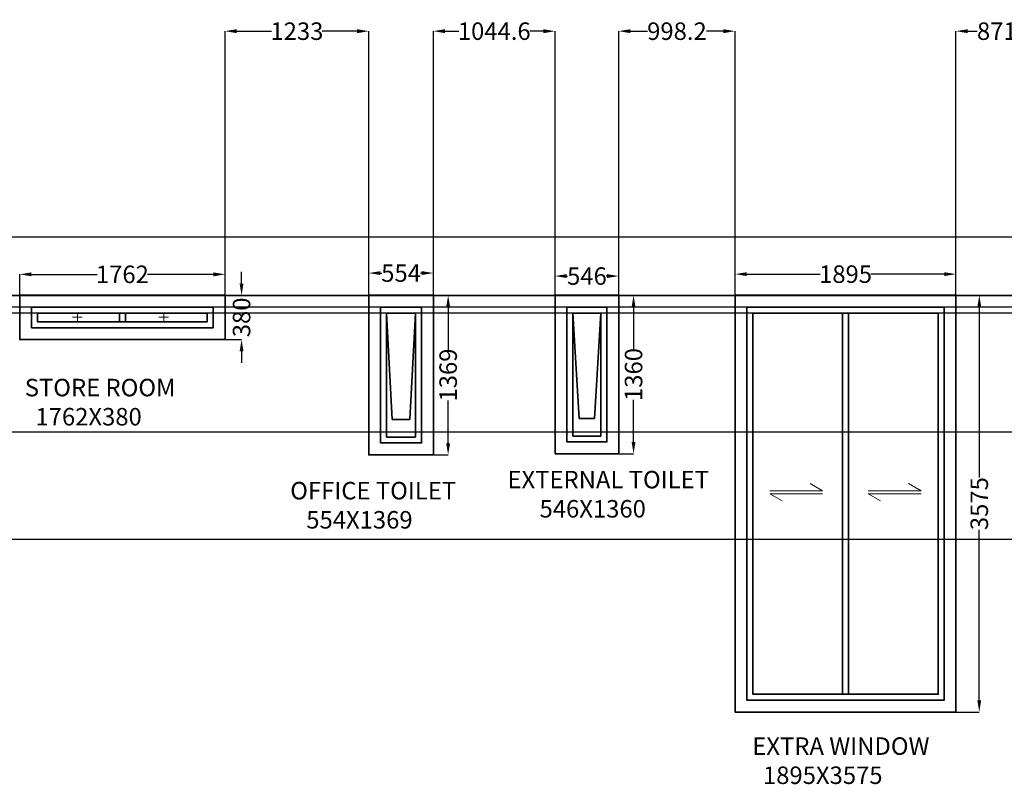
# Model space of a CAD drawing. Units: millimetres. Extents: x 16338 to 57165, y -4429 to 26237.
# Tile 3 of 6: x 32038 to 40486, y 2640 to 9199. Entities that reach past the tile are written whole.
import ezdxf

# ---------------------------------------------------------------- set-up
doc = ezdxf.new("R2010")
doc.units = ezdxf.units.MM
doc.header["$MEASUREMENT"] = 0
for name, color, linetype, lineweight in [('A-ANNO-DIMS', 5, 'Continuous', 18), ('A-ANNO-SYMB', 4, 'Continuous', 18), ('A-ANNO-TEXT', 3, 'Continuous', 18), ('A-ELEV', 8, 'Continuous', 25), ('A-GLAZ', 7, 'Continuous', 35)]:
    doc.layers.add(name, color=color, linetype=linetype, lineweight=lineweight)
doc.styles.get("Standard").update_dxf_attribs({"font": 'arial.ttf'})
doc.dimstyles.get("Standard").update_dxf_attribs({"dimtxt": 150, "dimasz": 100, "dimexe": 0.18, "dimexo": 0.0625, "dimgap": 0.09, "dimtad": 0, "dimdec": 0, "dimzin": 0, "dimdsep": 46, "dimtxsty": 'Standard', "dimcen": 0.09, "dimadec": 0, "dimazin": 0, "dimtfac": 1, "dimtdec": 0, "dimtofl": 0, "dimtmove": 0, "dimatfit": 3, "dimfxl": 1, "dimtolj": 1, "dimtzin": 0, "dimarcsym": 0})

# ---------------------------------------------------------------- blocks, each defined once
blk = doc.blocks.new('*D59')
at = {"layer": 'A-ANNO-DIMS', "color": 0, "lineweight": -2, "transparency": 16777216}
for p, q in [((32038.1, 6835.2), (32038.1, 7014.4)), ((32138.1, 7014.2), (32702.9, 7014.2)), ((33700.1, 7014.2), (33135.4, 7014.2)), ((33800.1, 6835.2), (33800.1, 7014.4))]:
    blk.add_line(p, q, dxfattribs=at)
at = {"layer": 'A-ANNO-DIMS', "color": 0, "transparency": 16777216}
for points in [[(32138.1, 7030.9), (32138.1, 6997.5), (32038.1, 7014.2)], [(33700.1, 7030.9), (33700.1, 6997.5), (33800.1, 7014.2)]]:
    blk.add_solid(points, dxfattribs=at)
at = {"layer": 'Defpoints', "color": 0, "transparency": 16777216}
for p in [(33800.1, 7014.2), (32038.1, 6835.1), (33800.1, 6835.1)]:
    blk.add_point(p, dxfattribs=at)
at = {"layer": 'A-ANNO-DIMS', "color": 0, "transparency": 16777216, "insert": (32919.1, 7014.2), "char_height": 150, "attachment_point": 5}
blk.add_mtext('\\A1;1762', dxfattribs=at)
blk = doc.blocks.new('*D60')
at = {"layer": 'A-ANNO-DIMS', "color": 0, "lineweight": -2, "transparency": 16777216}
for p, q in [((33941.5, 6935.1), (33941.5, 7035.1)), ((33800.2, 6835.1), (33941.7, 6835.1)), ((33800.2, 6455.1), (33941.7, 6455.1)), ((33941.5, 6355.1), (33941.5, 6255.1))]:
    blk.add_line(p, q, dxfattribs=at)
at = {"layer": 'A-ANNO-DIMS', "color": 0, "transparency": 16777216}
for points in [[(33924.9, 6935.1), (33958.2, 6935.1), (33941.5, 6835.1)], [(33924.9, 6355.1), (33958.2, 6355.1), (33941.5, 6455.1)]]:
    blk.add_solid(points, dxfattribs=at)
at = {"layer": 'Defpoints', "color": 0, "transparency": 16777216}
for p in [(33800.1, 6835.1), (33800.1, 6455.1), (33941.5, 6455.1)]:
    blk.add_point(p, dxfattribs=at)
at = {"layer": 'A-ANNO-DIMS', "color": 0, "transparency": 16777216, "insert": (33941.5, 6645.1), "char_height": 150, "attachment_point": 5, "rotation": 90}
blk.add_mtext('\\A1;380', dxfattribs=at)
blk = doc.blocks.new('*D61')
at = {"layer": 'A-ANNO-DIMS', "color": 0, "lineweight": -2, "transparency": 16777216}
for p, q in [((35033.2, 6835.2), (35033.2, 7025.4)), ((35133.2, 7025.2), (35144.7, 7025.2)), ((35487.2, 7025.2), (35475.7, 7025.2)), ((35587.2, 6835.2), (35587.2, 7025.4))]:
    blk.add_line(p, q, dxfattribs=at)
at = {"layer": 'A-ANNO-DIMS', "color": 0, "transparency": 16777216}
for points in [[(35133.2, 7041.9), (35133.2, 7008.5), (35033.2, 7025.2)], [(35487.2, 7041.9), (35487.2, 7008.5), (35587.2, 7025.2)]]:
    blk.add_solid(points, dxfattribs=at)
at = {"layer": 'Defpoints', "color": 0, "transparency": 16777216}
for p in [(35587.2, 7025.2), (35033.2, 6835.1), (35587.2, 6835.1)]:
    blk.add_point(p, dxfattribs=at)
at = {"layer": 'A-ANNO-DIMS', "color": 0, "transparency": 16777216, "insert": (35310.2, 7025.2), "char_height": 150, "attachment_point": 5}
blk.add_mtext('\\A1;554', dxfattribs=at)
blk = doc.blocks.new('*D62')
at = {"layer": 'A-ANNO-DIMS', "color": 0, "lineweight": -2, "transparency": 16777216}
for p, q in [((35587.2, 6835.1), (35714.3, 6835.1)), ((35714.1, 6735.1), (35714.1, 6367.8)), ((35714.1, 5566.1), (35714.1, 5933.4)), ((35587.2, 5466.1), (35714.3, 5466.1))]:
    blk.add_line(p, q, dxfattribs=at)
at = {"layer": 'A-ANNO-DIMS', "color": 0, "transparency": 16777216}
for points in [[(35697.5, 6735.1), (35730.8, 6735.1), (35714.1, 6835.1)], [(35697.5, 5566.1), (35730.8, 5566.1), (35714.1, 5466.1)]]:
    blk.add_solid(points, dxfattribs=at)
at = {"layer": 'Defpoints', "color": 0, "transparency": 16777216}
for p in [(35587.2, 6835.1), (35587.2, 5466.1), (35714.1, 5466.1)]:
    blk.add_point(p, dxfattribs=at)
at = {"layer": 'A-ANNO-DIMS', "color": 0, "transparency": 16777216, "insert": (35714.1, 6150.6), "char_height": 150, "attachment_point": 5, "rotation": 90}
blk.add_mtext('\\A1;1369', dxfattribs=at)
blk = doc.blocks.new('*D63')
at = {"layer": 'A-ANNO-DIMS', "color": 0, "lineweight": -2, "transparency": 16777216}
for p, q in [((36631.8, 6835.2), (36631.8, 6999.8)), ((36731.8, 6999.6), (36739, 6999.6)), ((37077.8, 6999.6), (37070.5, 6999.6)), ((37177.8, 6835.2), (37177.8, 6999.8))]:
    blk.add_line(p, q, dxfattribs=at)
at = {"layer": 'A-ANNO-DIMS', "color": 0, "transparency": 16777216}
for points in [[(36731.8, 7016.3), (36731.8, 6983), (36631.8, 6999.6)], [(37077.8, 7016.3), (37077.8, 6983), (37177.8, 6999.6)]]:
    blk.add_solid(points, dxfattribs=at)
at = {"layer": 'Defpoints', "color": 0, "transparency": 16777216}
for p in [(37177.8, 6999.6), (36631.8, 6835.1), (37177.8, 6835.1)]:
    blk.add_point(p, dxfattribs=at)
at = {"layer": 'A-ANNO-DIMS', "color": 0, "transparency": 16777216, "insert": (36904.8, 6999.6), "char_height": 150, "attachment_point": 5}
blk.add_mtext('\\A1;546', dxfattribs=at)
blk = doc.blocks.new('*D64')
at = {"layer": 'A-ANNO-DIMS', "color": 0, "lineweight": -2, "transparency": 16777216}
for p, q in [((37177.8, 6835.1), (37304.9, 6835.1)), ((37304.7, 6735.1), (37304.7, 6371.9)), ((37304.7, 5575.1), (37304.7, 5938.4)), ((37177.8, 5475.1), (37304.9, 5475.1))]:
    blk.add_line(p, q, dxfattribs=at)
at = {"layer": 'A-ANNO-DIMS', "color": 0, "transparency": 16777216}
for points in [[(37288, 6735.1), (37321.4, 6735.1), (37304.7, 6835.1)], [(37288, 5575.1), (37321.4, 5575.1), (37304.7, 5475.1)]]:
    blk.add_solid(points, dxfattribs=at)
at = {"layer": 'Defpoints', "color": 0, "transparency": 16777216}
for p in [(37177.8, 6835.1), (37177.8, 5475.1), (37304.7, 5475.1)]:
    blk.add_point(p, dxfattribs=at)
at = {"layer": 'A-ANNO-DIMS', "color": 0, "transparency": 16777216, "insert": (37304.7, 6155.1), "char_height": 150, "attachment_point": 5, "rotation": 90}
blk.add_mtext('\\A1;1360', dxfattribs=at)
blk = doc.blocks.new('*D65')
at = {"layer": 'A-ANNO-DIMS', "color": 0, "lineweight": -2, "transparency": 16777216}
for p, q in [((38176, 6835.2), (38176, 7016.2)), ((38276, 7016.1), (38905.9, 7016.1)), ((39971, 7016.1), (39341, 7016.1)), ((40071, 6835.2), (40071, 7016.2))]:
    blk.add_line(p, q, dxfattribs=at)
at = {"layer": 'A-ANNO-DIMS', "color": 0, "transparency": 16777216}
for points in [[(38276, 7032.7), (38276, 6999.4), (38176, 7016.1)], [(39971, 7032.7), (39971, 6999.4), (40071, 7016.1)]]:
    blk.add_solid(points, dxfattribs=at)
at = {"layer": 'Defpoints', "color": 0, "transparency": 16777216}
for p in [(40071, 7016.1), (38176, 6835.1), (40071, 6835.1)]:
    blk.add_point(p, dxfattribs=at)
at = {"layer": 'A-ANNO-DIMS', "color": 0, "transparency": 16777216, "insert": (39123.5, 7016.1), "char_height": 150, "attachment_point": 5}
blk.add_mtext('\\A1;1895', dxfattribs=at)
blk = doc.blocks.new('*D66')
at = {"layer": 'A-ANNO-DIMS', "color": 0, "lineweight": -2, "transparency": 16777216}
for p, q in [((40071, 6835.1), (40271.1, 6835.1)), ((40270.9, 6735.1), (40270.9, 5272.2)), ((40270.9, 3360.1), (40270.9, 4823)), ((40071, 3260.1), (40271.1, 3260.1))]:
    blk.add_line(p, q, dxfattribs=at)
at = {"layer": 'A-ANNO-DIMS', "color": 0, "transparency": 16777216}
for points in [[(40254.2, 6735.1), (40287.6, 6735.1), (40270.9, 6835.1)], [(40254.2, 3360.1), (40287.6, 3360.1), (40270.9, 3260.1)]]:
    blk.add_solid(points, dxfattribs=at)
at = {"layer": 'Defpoints', "color": 0, "transparency": 16777216}
for p in [(40071, 6835.1), (40071, 3260.1), (40270.9, 3260.1)]:
    blk.add_point(p, dxfattribs=at)
at = {"layer": 'A-ANNO-DIMS', "color": 0, "transparency": 16777216, "insert": (40270.9, 5047.6), "char_height": 150, "attachment_point": 5, "rotation": 90}
blk.add_mtext('\\A1;3575', dxfattribs=at)
blk = doc.blocks.new('SLIDE-ARROW-L')
for p, q in [((454.2, 0), (346.9, 62)), ((0, 0), (454.2, 0))]:
    blk.add_line(p, q)
blk = doc.blocks.new('*D113')
at = {"layer": 'A-ANNO-DIMS', "color": 0, "lineweight": -2, "transparency": 16777216}
for p, q in [((33800.1, 6835.2), (33800.1, 9100.3)), ((33900.1, 9100.1), (34199.6, 9100.1)), ((34933.2, 9100.1), (34633.7, 9100.1)), ((35033.2, 6835.2), (35033.2, 9100.3))]:
    blk.add_line(p, q, dxfattribs=at)
at = {"layer": 'A-ANNO-DIMS', "color": 0, "transparency": 16777216}
for points in [[(33900.1, 9116.8), (33900.1, 9083.4), (33800.1, 9100.1)], [(34933.2, 9116.8), (34933.2, 9083.4), (35033.2, 9100.1)]]:
    blk.add_solid(points, dxfattribs=at)
at = {"layer": 'Defpoints', "color": 0, "transparency": 16777216}
for p in [(35033.2, 9100.1), (33800.1, 6835.1), (35033.2, 6835.1)]:
    blk.add_point(p, dxfattribs=at)
at = {"layer": 'A-ANNO-DIMS', "color": 0, "transparency": 16777216, "insert": (34416.7, 9100.1), "char_height": 150, "attachment_point": 5}
blk.add_mtext('\\A1;1233', dxfattribs=at)
blk = doc.blocks.new('*D114')
at = {"layer": 'A-ANNO-DIMS', "color": 0, "lineweight": -2, "transparency": 16777216}
for p, q in [((35587.2, 6835.2), (35587.2, 9100.3)), ((35687.2, 9100.1), (35805.1, 9100.1)), ((36531.8, 9100.1), (36413.8, 9100.1)), ((36631.8, 6835.2), (36631.8, 9100.3))]:
    blk.add_line(p, q, dxfattribs=at)
at = {"layer": 'A-ANNO-DIMS', "color": 0, "transparency": 16777216}
for points in [[(35687.2, 9116.8), (35687.2, 9083.4), (35587.2, 9100.1)], [(36531.8, 9116.8), (36531.8, 9083.4), (36631.8, 9100.1)]]:
    blk.add_solid(points, dxfattribs=at)
at = {"layer": 'Defpoints', "color": 0, "transparency": 16777216}
for p in [(36631.8, 9100.1), (35587.2, 6835.1), (36631.8, 6835.1)]:
    blk.add_point(p, dxfattribs=at)
at = {"layer": 'A-ANNO-DIMS', "color": 0, "transparency": 16777216, "insert": (36109.5, 9100.1), "char_height": 150, "attachment_point": 5}
blk.add_mtext('\\A1;1044.6', dxfattribs=at)
blk = doc.blocks.new('*D115')
at = {"layer": 'A-ANNO-DIMS', "color": 0, "lineweight": -2, "transparency": 16777216}
for p, q in [((37177.8, 6835.2), (37177.8, 9100.3)), ((37277.8, 9100.1), (37424.5, 9100.1)), ((38076, 9100.1), (37929.3, 9100.1)), ((38176, 6835.2), (38176, 9100.3))]:
    blk.add_line(p, q, dxfattribs=at)
at = {"layer": 'A-ANNO-DIMS', "color": 0, "transparency": 16777216}
for points in [[(37277.8, 9116.8), (37277.8, 9083.4), (37177.8, 9100.1)], [(38076, 9116.8), (38076, 9083.4), (38176, 9100.1)]]:
    blk.add_solid(points, dxfattribs=at)
at = {"layer": 'Defpoints', "color": 0, "transparency": 16777216}
for p in [(38176, 9100.1), (37177.8, 6835.1), (38176, 6835.1)]:
    blk.add_point(p, dxfattribs=at)
at = {"layer": 'A-ANNO-DIMS', "color": 0, "transparency": 16777216, "insert": (37676.9, 9100.1), "char_height": 150, "attachment_point": 5}
blk.add_mtext('\\A1;998.2', dxfattribs=at)
blk = doc.blocks.new('*D116')
at = {"layer": 'A-ANNO-DIMS', "color": 0, "lineweight": -2, "transparency": 16777216}
for p, q in [((40071, 6835.2), (40071, 9100.3)), ((40171, 9100.1), (40254, 9100.1)), ((40842.1, 9100.1), (40759.1, 9100.1)), ((40942.1, 6834.3), (40942.1, 9100.3))]:
    blk.add_line(p, q, dxfattribs=at)
at = {"layer": 'A-ANNO-DIMS', "color": 0, "transparency": 16777216}
for points in [[(40171, 9116.8), (40171, 9083.4), (40071, 9100.1)], [(40842.1, 9116.8), (40842.1, 9083.4), (40942.1, 9100.1)]]:
    blk.add_solid(points, dxfattribs=at)
at = {"layer": 'Defpoints', "color": 0, "transparency": 16777216}
for p in [(40942.1, 9100.1), (40071, 6835.1), (40942.1, 6834.2)]:
    blk.add_point(p, dxfattribs=at)
at = {"layer": 'A-ANNO-DIMS', "color": 0, "transparency": 16777216, "insert": (40506.6, 9100.1), "char_height": 150, "attachment_point": 5}
blk.add_mtext('\\A1;871.2', dxfattribs=at)
blk = doc.blocks.new('*D126')
at = {"layer": 'A-ANNO-DIMS', "color": 0, "lineweight": -2, "transparency": 16777216}
for p, q in [((52647.9, 6935.1), (52647.9, 7035.1)), ((23824.7, 6835.1), (52648.1, 6835.1)), ((23724.7, 6735.1), (52648.1, 6735.1)), ((52647.9, 6635.1), (52647.9, 6535.1))]:
    blk.add_line(p, q, dxfattribs=at)
at = {"layer": 'A-ANNO-DIMS', "color": 0, "transparency": 16777216}
for points in [[(52631.2, 6935.1), (52664.6, 6935.1), (52647.9, 6835.1)], [(52631.2, 6635.1), (52664.6, 6635.1), (52647.9, 6735.1)]]:
    blk.add_solid(points, dxfattribs=at)
at = {"layer": 'Defpoints', "color": 0, "transparency": 16777216}
for p in [(23824.6, 6835.1), (23724.6, 6735.1), (52647.9, 6735.1)]:
    blk.add_point(p, dxfattribs=at)
at = {"layer": 'A-ANNO-DIMS', "color": 0, "transparency": 16777216, "insert": (52647.9, 6376.6), "char_height": 150, "attachment_point": 5, "rotation": 90}
blk.add_mtext('\\A1;100', dxfattribs=at)
blk = doc.blocks.new('*D127')
at = {"layer": 'A-ANNO-DIMS', "color": 0, "lineweight": -2, "transparency": 16777216}
for p, q in [((52647.9, 6835.1), (52647.9, 6935.1)), ((23673.9, 6684.3), (52648.1, 6684.3)), ((23724.7, 6735.1), (52648.1, 6735.1)), ((52647.9, 6584.3), (52647.9, 6484.3))]:
    blk.add_line(p, q, dxfattribs=at)
at = {"layer": 'A-ANNO-DIMS', "color": 0, "transparency": 16777216}
for points in [[(52631.2, 6835.1), (52664.6, 6835.1), (52647.9, 6735.1)], [(52631.2, 6584.3), (52664.6, 6584.3), (52647.9, 6684.3)]]:
    blk.add_solid(points, dxfattribs=at)
at = {"layer": 'Defpoints', "color": 0, "transparency": 16777216}
for p in [(23673.8, 6684.3), (23724.6, 6735.1), (52647.9, 6684.3)]:
    blk.add_point(p, dxfattribs=at)
at = {"layer": 'A-ANNO-DIMS', "color": 0, "transparency": 16777216, "insert": (52647.9, 6289.2), "char_height": 150, "attachment_point": 5, "rotation": 90}
blk.add_mtext('\\A1;50.8', dxfattribs=at)
blk = doc.blocks.new('*D132')
at = {"layer": 'A-ANNO-DIMS', "color": 0, "lineweight": -2, "transparency": 16777216}
for p, q in [((23673.9, 5663.2), (52648.1, 5663.2)), ((52647.9, 5563.2), (52647.9, 5441.3)), ((52647.9, 4842), (52647.9, 4963.9)), ((23615.6, 4742), (52648.1, 4742))]:
    blk.add_line(p, q, dxfattribs=at)
at = {"layer": 'A-ANNO-DIMS', "color": 0, "transparency": 16777216}
for points in [[(52631.2, 5563.2), (52664.6, 5563.2), (52647.9, 5663.2)], [(52631.2, 4842), (52664.6, 4842), (52647.9, 4742)]]:
    blk.add_solid(points, dxfattribs=at)
at = {"layer": 'Defpoints', "color": 0, "transparency": 16777216}
for p in [(23673.8, 5663.2), (52647.9, 5663.2), (23615.6, 4742)]:
    blk.add_point(p, dxfattribs=at)
at = {"layer": 'A-ANNO-DIMS', "color": 0, "transparency": 16777216, "insert": (52647.9, 5202.6), "char_height": 150, "attachment_point": 5, "rotation": 90}
blk.add_mtext('\\A1;921.1', dxfattribs=at)

msp = doc.modelspace()

# ---------------------------------------------------------------- linework, layer by layer
at = {"layer": 'A-ANNO-SYMB'}
for p, q in [((32492.52, 6645.62), (32575.1, 6645.62)), ((32533.81, 6615.33), (32533.81, 6672.29)), ((33232.11, 6645.62), (33314.69, 6645.62)), ((33273.4, 6615.33), (33273.4, 6672.29))]:
    msp.add_line(p, q, dxfattribs=at)
at = {"layer": 'A-ELEV'}
for p, q in [((18209.23, 7335.1), (50757.08, 7335.1)), ((18201.83, 6834.85), (50882.91, 6829.39))]:
    msp.add_line(p, q, dxfattribs=at)
at = {"layer": 'A-GLAZ'}
for p, q in [((32893.73, 6682.7), (32893.73, 6607.5)), ((32944.53, 6682.7), (32944.53, 6607.5)), ((35185.57, 6682.7), (35434.77, 6682.7)), ((35185.57, 5618.5), (35185.57, 6682.7)), ((35185.57, 6682.7), (35234.02, 5768.5)), ((35434.77, 6682.7), (35386.33, 5768.5)), ((35434.77, 6682.7), (35434.77, 5618.5)), ((36784.18, 6682.7), (37025.38, 6682.7)), ((36784.18, 5627.5), (36784.18, 6682.7)), ((36784.18, 6682.7), (36839.44, 5777.5)), ((37025.38, 6682.7), (36970.12, 5777.5)), ((37025.38, 6682.7), (37025.38, 5627.5)), ((39098.07, 6682.7), (39098.07, 3412.5)), ((39148.87, 6682.7), (39148.87, 3412.5)), ((35386.33, 5768.5), (35234.02, 5768.5)), ((36970.12, 5777.5), (36839.44, 5777.5)), ((35434.77, 5618.5), (35185.57, 5618.5)), ((37025.38, 5627.5), (36784.18, 5627.5))]:
    msp.add_line(p, q, dxfattribs=at)
for points in [[(32038.13, 6835.1), (33800.13, 6835.1), (33800.13, 6455.1), (32038.13, 6455.1)], [(35033.17, 6835.1), (35587.17, 6835.1), (35587.17, 5466.1), (35033.17, 5466.1)], [(36631.78, 6835.1), (37177.78, 6835.1), (37177.78, 5475.1), (36631.78, 5475.1)], [(38175.97, 6835.1), (40070.97, 6835.1), (40070.97, 3260.1), (38175.97, 3260.1)], [(32139.73, 6733.5), (33698.53, 6733.5), (33698.53, 6556.7), (32139.73, 6556.7)], [(32190.53, 6682.7), (33647.73, 6682.7), (33647.73, 6607.5), (32190.53, 6607.5)], [(35134.77, 6733.5), (35485.57, 6733.5), (35485.57, 5567.7), (35134.77, 5567.7)], [(36733.38, 6733.5), (37076.18, 6733.5), (37076.18, 5576.7), (36733.38, 5576.7)], [(38277.57, 6733.5), (39969.37, 6733.5), (39969.37, 3361.7), (38277.57, 3361.7)], [(38328.37, 6682.7), (39918.57, 6682.7), (39918.57, 3412.5), (38328.37, 3412.5)]]:
    msp.add_lwpolyline(points, close=True, dxfattribs=at)

# ---------------------------------------------------------------- block references
at = {"layer": 'A-ANNO-SYMB'}
for p in [(38472.73, 5156.9), (39316.72, 5156.9)]:
    msp.add_blockref('SLIDE-ARROW-L', p, dxfattribs=at)
at = {"layer": 'A-ANNO-SYMB', "rotation": 180}
for p in [(38926.93, 5132.25), (39770.92, 5132.25)]:
    msp.add_blockref('SLIDE-ARROW-L', p, dxfattribs=at)

# ---------------------------------------------------------------- texts
at = {"layer": 'A-ANNO-TEXT', "char_height": 150, "attachment_point": 1}
for s, insert in [('STORE ROOM\\P  1762X380', (32081.77, 6118.08)), ('EXTERNAL TOILET\\P      546X1360', (36223.1, 5328.43)), ('OFFICE TOILET\\P   554X1369', (34359.36, 5233.87)), ('EXTRA WINDOW\\P  1895X3575', (38323.32, 3042.82))]:
    msp.add_mtext_dynamic_manual_height_columns(s, width=7094.9176, gutter_width=1, heights=[0], dxfattribs=dict(at, insert=insert))

# ---------------------------------------------------------------- dimensions: what is measured, and where the dimension line sits
at = {"layer": 'A-ANNO-DIMS'}
for base, p1, p2, override, picture, middle in [((35033.17, 9100.1), (33800.13, 6835.1), (35033.17, 6835.1), {"dimdec": 0, "dimlfac": 1, "dimrnd": 0, "dimzin": 0, "dimdsep": 46, "dimlunit": 2}, '*D113', (34416.65, 9100.1)), ((36631.78, 9100.1), (35587.17, 6835.1), (36631.78, 6835.1), {"dimdec": 1, "dimlfac": 1, "dimrnd": 0, "dimzin": 0, "dimdsep": 46, "dimlunit": 2}, '*D114', (36109.48, 9100.1)), ((38175.97, 9100.1), (37177.78, 6835.1), (38175.97, 6835.1), {"dimdec": 1, "dimlfac": 1, "dimrnd": 0, "dimzin": 0, "dimdsep": 46, "dimlunit": 2}, '*D115', (37676.87, 9100.1)), ((40942.14, 9100.1), (40070.97, 6835.1), (40942.14, 6834.2), {"dimdec": 1, "dimlfac": 1, "dimrnd": 0, "dimzin": 0, "dimdsep": 46, "dimlunit": 2}, '*D116', (40506.55, 9100.1)), ((33800.13, 7014.2), (32038.13, 6835.1), (33800.13, 6835.1), {"dimclrd": 0, "dimclre": 0, "dimclrt": 0}, '*D59', (32919.13, 7014.2)), ((35587.17, 7025.19), (35033.17, 6835.1), (35587.17, 6835.1), {"dimclrd": 0, "dimclre": 0, "dimclrt": 0}, '*D61', (35310.17, 7025.19)), ((37177.78, 6999.64), (36631.78, 6835.1), (37177.78, 6835.1), {"dimclrd": 0, "dimclre": 0, "dimclrt": 0}, '*D63', (36904.78, 6999.64)), ((40070.97, 7016.05), (38175.97, 6835.1), (40070.97, 6835.1), {"dimclrd": 0, "dimclre": 0, "dimclrt": 0}, '*D65', (39123.47, 7016.05))]:
    dim = msp.add_linear_dim(base=base, p1=p1, p2=p2, dimstyle='Standard', override=override, dxfattribs=at)
    dim.commit()
    dim.dimension.update_dxf_attribs({"geometry": picture, "text_midpoint": middle})
for base, p1, p2, override, picture, middle in [((52647.91, 6735.1), (23824.59, 6835.1), (23724.59, 6735.1), {"dimdec": 0, "dimlfac": 1, "dimrnd": 0, "dimzin": 0, "dimdsep": 46, "dimlunit": 2}, '*D126', (52647.91, 6376.62)), ((33941.55, 6455.1), (33800.13, 6835.1), (33800.13, 6455.1), {"dimclrd": 0, "dimclre": 0, "dimclrt": 0}, '*D60', (33941.55, 6645.1)), ((52647.91, 6684.3), (23724.59, 6735.1), (23673.79, 6684.3), {"dimdec": 1, "dimlfac": 1, "dimrnd": 0, "dimzin": 0, "dimdsep": 46, "dimlunit": 2}, '*D127', (52647.91, 6289.25)), ((35714.12, 5466.1), (35587.17, 6835.1), (35587.17, 5466.1), {"dimclrd": 0, "dimclre": 0, "dimclrt": 0}, '*D62', (35714.12, 6150.6)), ((37304.7, 5475.1), (37177.78, 6835.1), (37177.78, 5475.1), {"dimclrd": 0, "dimclre": 0, "dimclrt": 0}, '*D64', (37304.7, 6155.1)), ((40270.89, 3260.1), (40070.97, 6835.1), (40070.97, 3260.1), {"dimclrd": 0, "dimclre": 0, "dimclrt": 0}, '*D66', (40270.89, 5047.6)), ((52647.91, 5663.17), (23615.55, 4742.04), (23673.79, 5663.17), {"dimdec": 1, "dimlfac": 1, "dimrnd": 0, "dimzin": 0, "dimdsep": 46, "dimlunit": 2}, '*D132', (52647.91, 5202.6))]:
    dim = msp.add_linear_dim(base=base, p1=p1, p2=p2, angle=90, dimstyle='Standard', override=override, dxfattribs=at)
    dim.commit()
    dim.dimension.update_dxf_attribs({"geometry": picture, "text_midpoint": middle})

doc.saveas('drawing.dxf')
